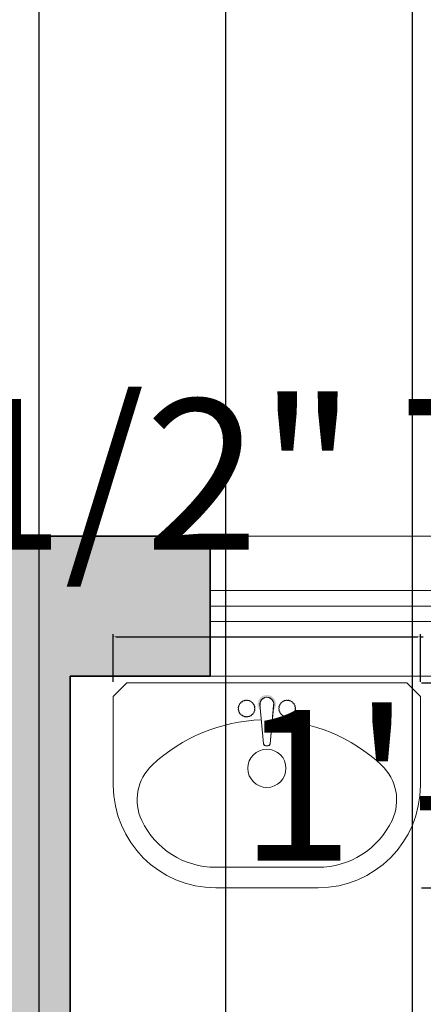
# Model space of a CAD drawing. Units: inches. Extents: x 2103 to 2702, y 2405 to 3142.
# Tile 5 of 7: x 2470 to 2496, y 3039 to 3102. Entities that reach past the tile are written whole.
import ezdxf

# ---------------------------------------------------------------- set-up
doc = ezdxf.new("R2010")
doc.units = ezdxf.units.IN
for name, color, linetype, lineweight in [('A-ANNO-DIMS', 2, 'Continuous', 18), ('A-FLOR-FIXT', 9, 'Continuous', 18), ('A-WALL-PATT', 8, 'Continuous', 9), ('WALL', 7, 'Continuous', 35), ('windows', 4, 'Continuous', 18)]:
    doc.layers.add(name, color=color, linetype=linetype, lineweight=lineweight)
doc.styles.get("Standard").update_dxf_attribs({"font": 'arial.ttf'})
doc.dimstyles.get("Standard").update_dxf_attribs({"dimtxt": 9.68, "dimasz": 0.18, "dimexe": 0.18, "dimexo": 0.0625, "dimgap": 0.09, "dimtad": 0, "dimtih": 1, "dimtoh": 1, "dimdec": 1, "dimzin": 0, "dimdsep": 46, "dimlunit": 3, "dimtxsty": 'Standard', "dimcen": 0.09, "dimadec": 0, "dimazin": 0, "dimtfac": 1, "dimtdec": 1, "dimtofl": 0, "dimtmove": 0, "dimatfit": 3, "dimfxl": 1, "dimtolj": 1, "dimtzin": 0, "dimarcsym": 0})

# ---------------------------------------------------------------- blocks, each defined once
blk = doc.blocks.new('ventilator')
at = {"layer": 'windows'}
for p, q in [((1922.124737122385, 2523.053655013118), (1898.124737122385, 2523.053655013118)), ((1922.124737122385, 2522.053655013118), (1898.124737122385, 2522.053655013118)), ((1922.124737122385, 2521.053655013119), (1898.124737122385, 2521.053655013119))]:
    blk.add_line(p, q, dxfattribs=at)
blk.add_lwpolyline([(1898.124737122385, 2526.553655012885), (1898.124737122385, 2517.553655012886), (1922.124737122385, 2517.553655013119), (1922.124737122385, 2526.553655013119)], close=True, dxfattribs=at)
blk = doc.blocks.new('s_46')
at = {"ltscale": 600}
h = blk.add_hatch(color=256, dxfattribs=at)
edge = h.paths.add_edge_path()
edge.add_line((13.45184378023259, 62.04360352296498), (14.15927104179718, 54.09782096462731))
edge.add_ellipse((4.212458010588306, 52.31250418393756), major_axis=(-10.10576298371302, 2.5e-15), ratio=1, start_angle=540, end_angle=550.1754626554052, ccw=False)
edge.add_arc((4.212458010588306, 52.31250418393756), 10.10576298371302, 270, 360, ccw=False)
edge.add_line((4.212458010588306, 42.20674120020703), (4.212458010588306, 41.28018079043977))
edge.add_line((4.212458010588306, 41.28018079040339), (11.85106942148559, 41.28018079040339))
edge.add_arc((4.212458010588306, 52.31250418393756), 13.41866400745597, 664.6981342835142, 766.4847699121552)
h.paths.add_polyline_path([(4.212458010588306, 41.28018079040339), (-3.426153400272596, 41.28018079040339, 0.152566653256377), (4.212458010588306, 38.8938401764608)])
h.paths.add_polyline_path([(11.85106942144921, 41.28018079040339), (4.212458010588306, 41.28018079040339), (4.212458010588306, 38.8938401764608, 0.1525666532563772)])
h.paths.add_polyline_path([(-5.734355020395014, 54.09782096461277), (-5.026927758881356, 62.04360352296498, 0.4758332592079194), (-3.426153400272596, 41.28018079040339), (4.212458010588306, 41.28018079040339), (4.212458010588306, 42.20674120020703, -0.4672400657637396)])
for p, q in [((-5.893304973142221, 52.31250418385025), (-0.714987907151226, 110.4750654234667)), ((-5.893304973142221, 52.31250418385025), (-0.714987907151226, 110.4750654234667)), ((9.139903928502463, 110.475065423554), (14.15927104174625, 54.09782096461277)), ((14.31822099431883, 52.31250418385025), (9.139903928502463, 110.475065423554)), ((14.15927104174625, 54.09782096461277), (14.31822099431883, 52.31250418385025))]:
    blk.add_line(p, q, dxfattribs=at)
blk.add_lwpolyline([(-220.7875419894117, 171.2801807903452, -0.4142135623730951), (-70.7875419894117, 321.2801807903452), (79.2124580105883, 321.2801807904325, -0.4142135623730951), (229.2124580105883, 171.2801807904325), (229.2124580105883, 41.28018079040339), (209.2124580107047, 21.2801807904325), (-200.7875419893535, 21.28018079034518), (-220.7875419894117, 41.28018079040339)], format="xyb", close=True, dxfattribs=at)
blk.add_lwpolyline([(12.26164246437838, 75.41187665969483, 0.1816379869150311), (172.1859176590806, 141.5383421540609, 0.3263505073803008), (187.6570333366981, 222.6589125997853, 0.2898144196813102), (79.21245801076293, 291.2801807904325), (-70.78754198923707, 291.2801807903452, 0.2898144196813102), (-179.2321173155214, 222.658912599698, 0.3263505073803008), (-163.7610016377293, 141.5383421540609, 0.1816379869150315), (-3.836726442852523, 75.41187665960751)], format="xyb", dxfattribs=at)
for points in [[(-16.83803374727722, 67.43055756771354), (-17.02338931558188, 67.50428807432763), (-17.22058725368697, 67.56961317334208), (-17.42189012444578, 67.6347039079701), (-17.61956049106084, 67.70773132116301), (-17.80586091603618, 67.79686645595939), (-17.97305396257434, 67.91028035557245), (-18.11578784312587, 68.05326030802098), (-18.23825336818117, 68.21955858168076), (-18.34702699835179, 68.40004368982045), (-18.44868519355077, 68.58558414605795), (-18.54980441438965, 68.76704846357461), (-18.65696112113073, 68.9353051558137), (-18.77673177386168, 69.08122273621848), (-18.91569283319404, 69.19566971814493), (-19.07841429975815, 69.27267628890695), (-19.26144033775199, 69.31891933156292), (-19.45930865121772, 69.34423740339116), (-19.66655694507062, 69.35846906132065), (-19.87772292352747, 69.37145286262967), (-20.08734429115429, 69.39302736415993), (-20.2899587523425, 69.43303112310241), (-20.48010401183274, 69.50130269664805), (-20.65391131333308, 69.60429419830325), (-20.81388605764368, 69.73491196823306), (-20.96412718523061, 69.8826759030926), (-21.10873363655992, 70.03710589953698), (-21.25180435174844, 70.18772185422131), (-21.39743827126222, 70.3240436638007), (-21.54973433539272, 70.43559122501756), (-21.71279148443137, 70.5118844343524), (-21.88955151231494, 70.54600451889564), (-22.07832762773614, 70.54527802669325), (-22.27627589285839, 70.52059283622657), (-22.4805523698451, 70.48283682571491), (-22.68831312085968, 70.44289787355228), (-22.89671420806553, 70.41166385821998), (-23.10291169380071, 70.40002265802468), (-23.30406164005399, 70.41886215136037), (-23.49802141042892, 70.4753938675276), (-23.68545357254334, 70.56212393892929), (-23.86772199510597, 70.66788214896224), (-24.04619054717477, 70.78149828102323), (-24.22222309763311, 70.89180211850908), (-24.39718351518968, 70.98762344472925), (-24.57243566872785, 71.05779204316786), (-24.74934342730558, 71.09113769704709), (-24.92903553397628, 71.08022740500746), (-25.11170022917213, 71.03257702605333), (-25.2972906283685, 70.95943963443278), (-25.48575984616764, 70.8720683044812), (-25.67706099752104, 70.7817161102721), (-25.87114719772944, 70.69963612605352), (-26.0679715613951, 70.63708142607356), (-26.26748720381875, 70.60530508466763), (-26.46941223740578, 70.61182491958607), (-26.67252476507565, 70.64921772302478), (-26.87536788737634, 70.70632503094384), (-27.07648470485583, 70.77198837930337), (-27.27441831788747, 70.8350493038015), (-27.46771182701923, 70.88434934031102), (-27.6549083327991, 70.90873002487933), (-27.83455093560042, 70.8970328932919), (-28.00620139669627, 70.84190539614065), (-28.17349611973623, 70.75121864315588), (-28.34109016874572, 70.63664965887438), (-28.51363860827405, 70.50987546765828), (-28.69579650234664, 70.38257309404435), (-28.89221891516354, 70.26641956248204), (-29.10756091127405, 70.17309189750813), (-29.3464775547036, 70.11426712348475), (-29.61160253512208, 70.0940409177856), (-29.89748404390411, 70.0861835690448), (-30.19664889771957, 70.05688401864609), (-30.50162391323829, 69.9723312081478), (-30.80493590747938, 69.79871407902101), (-31.09911169676343, 69.50222157256212), (-31.37667809793493, 69.0490426304168), (-31.63016192783834, 68.40536619405611), (-32.32050594605971, 68.4500712644367), (-32.84873653826071, 68.3918758847285), (-33.24226493795868, 68.25193804170704), (-33.52850237919483, 68.0514157223224), (-33.73486009566113, 67.8114669136994), (-33.88874932087492, 67.5532496026135), (-34.01758128887741, 67.29792177610216), (-34.14876723336056, 67.06664142102818), (-34.30371923936764, 66.87550954936887), (-34.47985279804561, 66.72039927294827), (-34.66858425136889, 66.59212672835565), (-34.86132994201034, 66.48150805244222), (-35.04950621211901, 66.37935938188457), (-35.22452940384392, 66.27649685335928), (-35.37781585985795, 66.16373660371755), (-35.50078192248475, 66.03189476963598), (-35.58785390376579, 65.87432967920904), (-35.64549799636007, 65.69456842611542), (-35.68319036299363, 65.49868029527715), (-35.7104071660433, 65.2927345718781), (-35.73662456823513, 65.08280054092756), (-35.77131873212056, 64.87494748734753), (-35.82396582007641, 64.67524469623459), (-35.90404199482873, 64.48976145259803), (-36.01774371694773, 64.3227640100813), (-36.15814863995183, 64.17130649695173), (-36.31505471485434, 64.0306400101108), (-36.47825989319244, 63.89601564637269), (-36.63756212632871, 63.76268450255157), (-36.78275936545106, 63.62589767554891), (-36.90364956192207, 63.48090626226621), (-36.99003066710429, 63.32296135951764), (-37.03518227743916, 63.14869254492805), (-37.04631056915969, 62.96024331927765), (-37.03410336375237, 62.7611356638954), (-37.00924848217983, 62.55489156045951), (-36.98243374592858, 62.34503299021162), (-36.96434697631048, 62.13508193491725), (-36.96567599463743, 61.92856037581805), (-36.99710862222128, 61.72899029450491), (-37.06570762058254, 61.53896291530691), (-37.16403551277472, 61.35734643402975), (-37.28102976223454, 61.18207828939194), (-37.40562783187488, 61.0110959201993), (-37.52676718513249, 60.84233676508302), (-37.63338528544409, 60.67373826284892), (-37.7144195958972, 60.50323785204091), (-37.75880757992855, 60.32877297155209), (-37.75920177751686, 60.14875038337777), (-37.72311503690435, 59.96345414296957), (-37.66177528270055, 59.77363762940512), (-37.58641044021351, 59.58005422132555), (-37.5082484340528, 59.38345729780849), (-37.43851718935184, 59.18460023758234), (-37.38844463089481, 58.98423641963745), (-37.36925868364051, 58.78311922278953), (-37.38844463089481, 58.58200202594161), (-37.43851718935184, 58.38163820799673), (-37.5082484340528, 58.18278114777058), (-37.58641044021351, 57.98618422425352), (-37.66177528287517, 57.79260081626126), (-37.72311503690435, 57.6027843026095), (-37.75920177751686, 57.4174880622013), (-37.75880757992855, 57.23746547402697), (-37.7144195958972, 57.06300059353816), (-37.63338528544409, 56.89250018273014), (-37.52676718530711, 56.72390168049606), (-37.40562783187488, 56.55514252537978), (-37.28102976223454, 56.38416015618713), (-37.16403551277472, 56.20889201154932), (-37.06570762058254, 56.02727553035947), (-36.99710862222128, 55.83724815107416), (-36.96567599463743, 55.63767806976102), (-36.96434697631048, 55.43115651066182), (-36.98243374592858, 55.22120545536745), (-37.00924848217983, 55.01134688520687), (-37.03410336375237, 54.80510278168367), (-37.04631056933431, 54.60599512638873), (-37.03518227743916, 54.41754590065102), (-36.99003066710429, 54.24327708606142), (-36.90364956192207, 54.08533218331285), (-36.78275936545106, 53.94034077003016), (-36.63756212632871, 53.80355394302751), (-36.47825989319244, 53.67022279920639), (-36.31505471502896, 53.53559843546827), (-36.15814863995183, 53.39493194862734), (-36.01774371712236, 53.24347443549777), (-35.90404199482873, 53.07647699298104), (-35.82396582007641, 52.89099374934449), (-35.77131873212056, 52.69129095823155), (-35.73662456823513, 52.48343790465151), (-35.71040716621792, 52.27350387370098), (-35.68319036299363, 52.06755815021461), (-35.64549799653469, 51.87167001946363), (-35.58785390376579, 51.69190876637003), (-35.50078192248475, 51.53434367594309), (-35.3778353385278, 51.40284301002975), (-35.22468523163116, 51.29247093791491), (-35.05003213009331, 51.19609060572111), (-34.86257656256203, 51.10656515930895), (-34.67101905716118, 51.01675774488831), (-34.48406014236389, 50.91953150840708), (-34.31040034646867, 50.80774959607516), (-34.15874019777402, 50.67427515375311), (-34.03505195630714, 50.51453334218241), (-33.93439480883535, 50.3341973797942), (-33.84909967368003, 50.14150249981321), (-33.77149746881332, 49.94468393520219), (-33.69391911290586, 49.75197691909852), (-33.60869552427903, 49.57161668455228), (-33.50815762107959, 49.41183846470085), (-33.38463632145431, 49.28087749250699), (-33.23284944484476, 49.18408373402781), (-33.05706241185544, 49.11526608630083), (-32.86392754490953, 49.06534817945794), (-32.66009716555709, 49.02525364354369), (-32.45222359569743, 48.98590610860265), (-32.24695915722987, 48.93822920459206), (-32.05095617187908, 48.87314656155649), (-31.870866961719, 48.78158180962782), (-31.71133844077122, 48.65761859554914), (-31.5689958925941, 48.50798063381808), (-31.43845919286832, 48.34255165536887), (-31.31434821744915, 48.17121539139771), (-31.19128284219187, 48.00385557310073), (-31.06388294277713, 47.85035593167413), (-30.92676839523483, 47.72060019822674), (-30.77455907507101, 47.62447210386745), (-30.60346923320321, 47.56846716045401), (-30.41609062027419, 47.54552800310193), (-30.21660936163971, 47.54520904741366), (-30.00921158283018, 47.55706470907898), (-29.79808340937598, 47.570649403875), (-29.58741096680751, 47.57551754757878), (-29.38138038065517, 47.56122355579281), (-29.18417777627474, 47.51732184420689), (-28.99883273948217, 47.43692629240103), (-28.8237486963626, 47.32738863455597), (-28.65617253311211, 47.19962006882997), (-28.49335113610141, 47.06453179311938), (-28.33253139152657, 46.9330350055825), (-28.1709601857583, 46.81604090429027), (-28.00588440499268, 46.72446068713907), (-27.83455093577504, 46.66920555219985), (-27.6549083327991, 46.65750842061243), (-27.46771182701923, 46.68188910518074), (-27.27441831788747, 46.73118914177758), (-27.07648470485583, 46.7942500662757), (-26.87536788755096, 46.85991341454792), (-26.67252476525027, 46.91702072246698), (-26.4694122375804, 46.95441352590569), (-26.26748720399337, 46.96093336082412), (-26.06797156156972, 46.9291570194182), (-25.87114719772944, 46.86660231943824), (-25.67706099769566, 46.78452233530697), (-25.48575984616764, 46.69417014101054), (-25.2972906283685, 46.60679881105898), (-25.11170022934675, 46.53366141943843), (-24.92903553397628, 46.4860110404843), (-24.74934342730558, 46.47510074844467), (-24.57243566890247, 46.50844640232389), (-24.39718351536431, 46.57861500076251), (-24.22222309780773, 46.67443632698268), (-24.0461905473494, 46.78474016446853), (-23.86772199528059, 46.89835629652953), (-23.68545357254334, 47.00411450656247), (-23.49802141060354, 47.09084457796416), (-23.30406164022861, 47.14737629413138), (-23.10291169380071, 47.16621578746708), (-22.89671420806553, 47.15457458727178), (-22.68831312085968, 47.12334057193948), (-22.4805523698451, 47.08340161977685), (-22.27627589285839, 47.04564560926519), (-22.07832762791077, 47.02096041871118), (-21.88955151248956, 47.02023392650881), (-21.71279148443137, 47.05435401113937), (-21.54973433539272, 47.1306472204742), (-21.39743827126222, 47.24219478160375), (-21.25180435174844, 47.37851659118314), (-21.10873363655992, 47.52913254586746), (-20.96412718540523, 47.68356254231185), (-20.81388605764368, 47.83132647717138), (-20.65391131333308, 47.9619442471012), (-20.48010401200736, 48.0649357488437), (-20.28995875251712, 48.13320732230204), (-20.08734429115429, 48.17321108133183), (-19.87772292352747, 48.1947855828621), (-19.66655694507062, 48.2077693840838), (-19.45930865139235, 48.2220010421006), (-19.26144033775199, 48.24731911384152), (-19.07841429993277, 48.29356215667212), (-18.91569283319404, 48.37056872743414), (-18.77673177403631, 48.48501570936059), (-18.65696112113073, 48.63093328976538), (-18.54980441456428, 48.79918998200446), (-18.44868519372539, 48.98065429960843), (-18.34702699835179, 49.16619475575862), (-18.2382533683558, 49.34667986398562), (-18.11578784312587, 49.5129781376454), (-17.97305396274896, 49.6559580900066), (-17.8058609162108, 49.76937198961969), (-17.61956049106084, 49.85850712450337), (-17.4218901246204, 49.93153453769628), (-17.22058725368697, 49.996625272237), (-17.02338931558188, 50.06195037133875), (-16.83803374727722, 50.13568087795284), (-16.67225798609434, 50.22598783511785), (-16.53379946883069, 50.34104228604701), (-16.42766593385022, 50.48645191569812), (-16.34794632298872, 50.65757097714231), (-16.28599987912457, 50.84719036528259), (-16.23318584513618, 51.04810097528389), (-16.18086346407654, 51.25309370196191), (-16.12039197882404, 51.45495944039431), (-16.04313063243171, 51.64648908557137), (-15.94043866742868, 51.82047353248345), (-15.8067031877581, 51.97190354572376), (-15.64842273970134, 52.10456936812261), (-15.47512373042991, 52.22446111202589), (-15.29633256676607, 52.33756888969219), (-15.12157565605594, 52.44988281364204), (-14.96037940529641, 52.567392996134), (-14.82227022130973, 52.69608954960131), (-14.71677451161667, 52.84196258638985), (-14.6501372611965, 53.00919824198354), (-14.61547776852967, 53.19476674450561), (-14.60263391025364, 53.3938343450427), (-14.60144356318051, 53.60156729485606), (-14.60174460412236, 53.81313184503233), (-14.59337490954203, 54.02369424700736), (-14.566172356077, 54.22842075169319), (-14.50997482053935, 54.42247761052567), (-14.41809999983525, 54.6024088327249), (-14.29778487142175, 54.77026946117985), (-14.1597462335485, 54.92949229647638), (-14.01470088359201, 55.08351013963693), (-13.87336561962729, 55.23575579150929), (-13.7464572393801, 55.38966205302859), (-13.64469254092546, 55.54866172495531), (-13.5787883218145, 55.71618760822457), (-13.55583441938506, 55.89474125843844), (-13.56841282837558, 56.08309925056528), (-13.60547858278733, 56.27910691397847), (-13.65598671662155, 56.48060957840062), (-13.70889226370491, 56.68545257346704), (-13.7531502583879, 56.89148122872575), (-13.7777157346718, 57.09654087381204), (-13.77154372638324, 57.29847683827393), (-13.72730239736847, 57.49560352915432), (-13.65251243085367, 57.68811166286468), (-13.55840763938613, 57.8766610333987), (-13.45622183586238, 58.06191143448813), (-13.35718883317895, 58.24452266012667), (-13.27254244388314, 58.42515450413339), (-13.2135164810461, 58.60446676041465), (-13.19134475721512, 58.78311922278953), (-13.2135164810461, 58.96177168516442), (-13.27254244388314, 59.14108394144569), (-13.35718883317895, 59.3217157854524), (-13.45622183586238, 59.50432701109093), (-13.55840763938613, 59.68957741218037), (-13.65251243085367, 59.87812678271438), (-13.72730239736847, 60.07063491642475), (-13.77154372638324, 60.26776160730515), (-13.7777157346718, 60.46969757176703), (-13.7531502583879, 60.67475721685332), (-13.70889226370491, 60.88078587211203), (-13.65598671662155, 61.08562886717845), (-13.60547858278733, 61.2871315316006), (-13.56841282837558, 61.48313919501379), (-13.55583441938506, 61.67149718714063), (-13.5787883218145, 61.8500508373545), (-13.64469254092546, 62.01757672062377), (-13.7464572393801, 62.17657639255048), (-13.87336561962729, 62.33048265406978), (-14.01470088359201, 62.48272830594214), (-14.15974623337388, 62.63674614910269), (-14.29778487142175, 62.79596898448653), (-14.41809999983525, 62.96382961285416), (-14.50997482053935, 63.14376083514071), (-14.566172356077, 63.33781769388588), (-14.59337490936741, 63.5425441985717), (-14.60174460412236, 63.75310660054674), (-14.60144356318051, 63.96467115081032), (-14.60263391025364, 64.17240410053635), (-14.61547776835505, 64.37147170116077), (-14.65013726102188, 64.55704020359553), (-14.71677451144205, 64.7242758591892), (-14.82227022130973, 64.87014889597776), (-14.96037940529641, 64.99884544944507), (-15.12157565605594, 65.11635563193704), (-15.29633256676607, 65.22866955588688), (-15.47512373042991, 65.3417773336405), (-15.64842273970134, 65.46166907745646), (-15.8067031877581, 65.59433489985531), (-15.94043866742868, 65.74576491309563), (-16.04313063225709, 65.9197493600077), (-16.12039197882404, 66.11127900527208), (-16.18086346407654, 66.31314474370447), (-16.23318584513618, 66.5181374703825), (-16.28599987912457, 66.71904808029649), (-16.34794632298872, 66.90866746843676), (-16.42766593385022, 67.07978652988095), (-16.53379946883069, 67.22519615953206), (-16.67225798609434, 67.34025061046123)], [(22.08090273779817, 61.08562886709115), (22.03039460413856, 61.2871315315133), (21.99332884972682, 61.48313919501379), (21.9807504407363, 61.67149718705331), (22.00370434316574, 61.85005083726719), (22.06960856210208, 62.01757672053645), (22.17137326073134, 62.17657639246318), (22.29828164080391, 62.33048265398247), (22.43961690476863, 62.48272830585483), (22.58466225472512, 62.63674614901538), (22.72270089277299, 62.79596898439923), (22.84301602118649, 62.96382961276686), (22.93489084189059, 63.1437608350534), (22.99108837742824, 63.33781769379857), (23.01829093071865, 63.5425441985717), (23.0266606254736, 63.75310660045943), (23.02635958453175, 63.96467115072301), (23.02754993160488, 64.17240410053635), (23.04039378970629, 64.37147170107346), (23.07505328237312, 64.55704020350822), (23.14169053279329, 64.72427585910191), (23.24718624266097, 64.87014889589045), (23.38529542664764, 64.99884544935776), (23.54649167740717, 65.11635563193704), (23.7212485881173, 65.22866955579956), (23.90003975178115, 65.34177733355318), (24.07333876105258, 65.46166907736915), (24.23161920910934, 65.594334899768), (24.36535468877992, 65.74576491300832), (24.46804665360833, 65.9197493600077), (24.54530800017528, 66.11127900518477), (24.60577948542777, 66.31314474361714), (24.65810186648742, 66.51813747029519), (24.71091590047581, 66.71904808020918), (24.77286234433996, 66.90866746834945), (24.85258195520146, 67.07978652979364), (24.95871549018193, 67.22519615953206), (25.09717400744558, 67.34025061046123), (25.26294976862846, 67.43055756771354), (25.44830533693312, 67.50428807432763), (25.64550327503821, 67.56961317334208), (25.84680614579702, 67.6347039079701), (26.04447651241208, 67.70773132116301), (26.23077693756204, 67.79686645595939), (26.3979699841002, 67.91028035557245), (26.54070386447711, 68.05326030802098), (26.66316938970704, 68.21955858168076), (26.77194301970303, 68.40004368982045), (26.87360121507663, 68.58558414605795), (26.97472043591552, 68.76704846357461), (27.08187714248197, 68.9353051558137), (27.20164779538754, 69.08122273621848), (27.34060885454528, 69.19566971814493), (27.50333032128401, 69.27267628890695), (27.68635635910323, 69.31891933165025), (27.88422467274358, 69.34423740347847), (28.09147296642186, 69.35846906140794), (28.30263894487871, 69.37145286262967), (28.51226031250553, 69.39302736424725), (28.71487477386836, 69.43303112318972), (28.90502003318398, 69.50130269673537), (29.07882733468432, 69.60429419839056), (29.23880207899492, 69.73491196832038), (29.38904320658185, 69.88267590317992), (29.53364965791116, 70.0371058996243), (29.67672037309967, 70.18772185430862), (29.82235429261346, 70.324043663888), (29.97465035674395, 70.43559122501756), (30.1377075057826, 70.51188443443971), (30.31446753366618, 70.54600451898295), (30.50324364908738, 70.54527802678058), (30.70119191420963, 70.52059283622657), (30.90546839119634, 70.48283682571491), (31.11322914221091, 70.4428978736396), (31.32163022941677, 70.41166385830729), (31.52782771515195, 70.400022658112), (31.72897766157985, 70.41886215144768), (31.92293743178016, 70.4753938675276), (32.11036959389458, 70.56212393892929), (32.29263801663183, 70.66788214896224), (32.47110656870063, 70.78149828102323), (32.64713911898434, 70.89180211850908), (32.82209953654092, 70.98762344481656), (32.99735169025371, 71.05779204316786), (33.17425944865681, 71.09113769704709), (33.35395155532751, 71.08022740500746), (33.53661625069799, 71.03257702605333), (33.72220664971974, 70.9594396345201), (33.91067586751888, 70.8720683044812), (34.1019770190469, 70.7817161102721), (34.29606321908068, 70.69963612605352), (34.49288758292096, 70.63708142616088), (34.69240322534461, 70.60530508466763), (34.89432825893164, 70.61182491958607), (35.09744078660151, 70.64921772302478), (35.3002839089022, 70.70632503103116), (35.50140072620707, 70.77198837930337), (35.6993343392387, 70.8350493038015), (35.89262784837047, 70.88434934039833), (36.07982435415034, 70.90873002487933), (36.25946695695166, 70.8970328932919), (36.43111741804751, 70.84190539614065), (36.59841214108747, 70.75121864315588), (36.76600619009696, 70.63664965887438), (36.93855462962529, 70.50987546765828), (37.12071252369788, 70.38257309404435), (37.3171349366894, 70.26641956248204), (37.53247693262529, 70.17309189750813), (37.77139357605483, 70.11426712348475), (38.03651855647331, 70.0940409177856), (38.32240006525535, 70.0861835690448), (38.62156491907081, 70.05688401864609), (38.92653993476415, 69.9723312081478), (39.22985192883061, 69.79871407893368), (39.52402771811467, 69.50222157256212), (39.80159411928616, 69.0490426304168), (40.05507794918957, 68.4053661939688), (40.74542196741094, 68.4500712644367), (41.27365255961194, 68.3918758846412), (41.66718095948453, 68.25193804161972), (41.95341840054607, 68.0514157223224), (42.15977611701236, 67.8114669136121), (42.31366534240078, 67.5532496025262), (42.44249731022864, 67.29792177601485), (42.57368325471179, 67.06664142094087), (42.72863526071887, 66.87550954936887), (42.90476881939684, 66.72039927286096), (43.09350027272012, 66.59212672826834), (43.28624596336157, 66.48150805235491), (43.47442223347025, 66.37935938179726), (43.64944542536977, 66.27649685335928), (43.80273188138381, 66.16373660371755), (43.92569794383598, 66.03189476963598), (44.01276992511703, 65.87432967912173), (44.0704140177113, 65.69456842602813), (44.10810638434486, 65.49868029527715), (44.13532318739453, 65.2927345718781), (44.16154058958636, 65.08280054084025), (44.19623475347179, 64.87494748726021), (44.24888184142765, 64.67524469614727), (44.32895801617997, 64.48976145251072), (44.44265973829897, 64.32276400999397), (44.58306466130307, 64.17130649695173), (44.73997073620558, 64.03064001002348), (44.90317591454368, 63.89601564628538), (45.06247814767994, 63.76268450246425), (45.20767538680229, 63.6258976754616), (45.3285655832733, 63.4809062621789), (45.41494668845553, 63.32296135943034), (45.46009829879039, 63.14869254484074), (45.47122659051092, 62.96024331919034), (45.45901938492898, 62.76113566380809), (45.43416450353106, 62.5548915603722), (45.40734976727981, 62.34503299021162), (45.38926299766171, 62.13508193482994), (45.39059201598866, 61.92856037573074), (45.42202464357251, 61.7289902944176), (45.49062364193377, 61.53896291521959), (45.58895153412595, 61.35734643394243), (45.70594578341115, 61.18207828939194), (45.83054385322611, 61.01109592011198), (45.95168320648371, 60.84233676508302), (46.05830130679533, 60.67373826276162), (46.13933561724843, 60.50323785204091), (46.18372360127978, 60.32877297146479), (46.1841177988681, 60.14875038329046), (46.14803105825558, 59.96345414296957), (46.08669130405178, 59.77363762931782), (46.01132646156474, 59.58005422123824), (45.93316445540404, 59.38345729772118), (45.86343321070308, 59.18460023749503), (45.81336065224604, 58.98423641955014), (45.79417470499175, 58.78311922270222), (45.81336065224604, 58.58200202585431), (45.86343321070308, 58.38163820790942), (45.93316445540404, 58.18278114777058), (46.01132646156474, 57.98618422416621), (46.08669130405178, 57.79260081617394), (46.14803105808095, 57.6027843025222), (46.1841177988681, 57.4174880622013), (46.18372360127978, 57.23746547393966), (46.13933561724843, 57.06300059345085), (46.05830130679533, 56.89250018273014), (45.95168320648371, 56.72390168040874), (45.83054385322611, 56.55514252529247), (45.70594578341115, 56.38416015609982), (45.58895153412595, 56.20889201154932), (45.49062364193377, 56.02727553027216), (45.42202464339789, 55.83724815107416), (45.39059201598866, 55.63767806976102), (45.38926299766171, 55.43115651066182), (45.40734976727981, 55.22120545528014), (45.43416450335644, 55.01134688511957), (45.45901938492898, 54.80510278159636), (45.47122659051092, 54.60599512630142), (45.46009829879039, 54.41754590056371), (45.41494668845553, 54.24327708597411), (45.32856558309868, 54.08533218322554), (45.20767538662767, 53.94034076994285), (45.06247814750532, 53.8035539429402), (44.90317591454368, 53.67022279920639), (44.73997073620558, 53.53559843538096), (44.58306466130307, 53.39493194854004), (44.44265973829897, 53.24347443541046), (44.32895801617997, 53.07647699298104), (44.24888184125302, 52.89099374934449), (44.19623475329717, 52.69129095823155), (44.16154058958636, 52.48343790465151), (44.13532318739453, 52.27350387361366), (44.10810638434486, 52.06755815021461), (44.0704140177113, 51.87167001946363), (44.01276992511703, 51.69190876628272), (43.92569794366136, 51.53434367585578), (43.80275135970442, 51.40284301002975), (43.64960125280776, 51.29247093791491), (43.47494815144455, 51.1960906056338), (43.28749258373863, 51.10656515922165), (43.09593507851241, 51.01675774480099), (42.90897616371512, 50.91953150840708), (42.73531636764528, 50.80774959598784), (42.58365621895063, 50.67427515375311), (42.45996797765838, 50.51453334218241), (42.35931083018658, 50.3341973797942), (42.27401569485664, 50.14150249981321), (42.19641349016455, 49.94468393520219), (42.1188351342571, 49.75197691909852), (42.03361154545564, 49.57161668455228), (41.9330736422562, 49.41183846461354), (41.80955234280554, 49.28087749250699), (41.65776546602137, 49.1840837339405), (41.48197843320668, 49.11526608630083), (41.28884356608614, 49.06534817945794), (41.0850131867337, 49.02525364354369), (40.87713961687405, 48.98590610851534), (40.67187517840648, 48.93822920459206), (40.47587219323031, 48.87314656155649), (40.29578298289561, 48.78158180962782), (40.13625446194782, 48.65761859554914), (39.99391191377072, 48.50798063373076), (39.86337521404493, 48.34255165528157), (39.73926423862577, 48.17121539139771), (39.61619886336848, 48.00385557310073), (39.48879896395374, 47.85035593167413), (39.35168441641144, 47.72060019813944), (39.19947509624762, 47.62447210378013), (39.02838525455445, 47.56846716045401), (38.8410066414508, 47.54552800310193), (38.64152538281633, 47.54520904732635), (38.43412760400679, 47.55706470907898), (38.22299943072721, 47.570649403875), (38.01232698798413, 47.57551754757878), (37.80629640183179, 47.56122355579281), (37.60909379745135, 47.51732184420689), (37.42374876065878, 47.43692629240103), (37.24866471753922, 47.32738863455597), (37.08108855428873, 47.19962006882997), (36.91826715727803, 47.06453179311938), (36.75744741270319, 46.9330350056698), (36.59587620693492, 46.81604090429027), (36.4308004261693, 46.72446068713907), (36.25946695695166, 46.66920555228716), (36.07982435397571, 46.65750842061243), (35.89262784837047, 46.68188910518074), (35.6993343392387, 46.73118914177758), (35.50140072620707, 46.7942500662757), (35.30028390872758, 46.85991341454792), (35.09744078642689, 46.91702072246698), (34.89432825875701, 46.954413525993), (34.69240322516998, 46.96093336082412), (34.49288758274633, 46.9291570194182), (34.29606321908068, 46.86660231943824), (34.10197701887228, 46.78452233530697), (33.91067586734425, 46.69417014109785), (33.72220664971974, 46.60679881105898), (33.53661625052337, 46.53366141943843), (33.35395155515289, 46.4860110404843), (33.17425944865681, 46.47510074844467), (32.99735169007909, 46.5084464024112), (32.82209953654092, 46.57861500076251), (32.64713911898434, 46.67443632707), (32.47110656852601, 46.78474016446853), (32.2926380164572, 46.89835629661684), (32.11036959389458, 47.00411450664979), (31.92293743178016, 47.09084457805147), (31.72897766140522, 47.14737629413138), (31.52782771497732, 47.16621578746708), (31.32163022941677, 47.15457458727178), (31.11322914203629, 47.12334057193948), (30.90546839102171, 47.08340161986416), (30.70119191420963, 47.0456456093525), (30.50324364908738, 47.02096041879849), (30.31446753366618, 47.02023392659611), (30.1377075057826, 47.05435401113937), (29.97465035674395, 47.13064722056151), (29.82235429261346, 47.24219478169106), (29.67672037309967, 47.37851659127045), (29.53364965791116, 47.52913254595478), (29.38904320658185, 47.68356254239916), (29.2388020788203, 47.8313264772587), (29.0788273345097, 47.96194424718851), (28.90502003318398, 48.06493574893102), (28.71487477369374, 48.13320732238935), (28.51226031250553, 48.17321108133183), (28.30263894487871, 48.19478558294941), (28.09147296642186, 48.20776938417111), (27.88422467256896, 48.22200104218791), (27.68635635892861, 48.24731911392882), (27.50333032110939, 48.29356215667212), (27.34060885454528, 48.37056872743414), (27.20164779521292, 48.48501570936059), (27.08187714248197, 48.63093328976538), (26.97472043574089, 48.79918998200446), (26.87360121490201, 48.98065429960843), (26.77194301952841, 49.16619475575862), (26.66316938953241, 49.34667986398562), (26.54070386447711, 49.51297813755809), (26.39796998392558, 49.6559580900066), (26.23077693738742, 49.76937198961969), (26.04447651223745, 49.85850712450337), (25.84680614579702, 49.93153453769628), (25.64550327486359, 49.996625272237), (25.44830533675849, 50.06195037133875), (25.26294976862846, 50.13568087795284), (25.09717400727095, 50.22598783520516), (24.95871549018193, 50.34104228604701), (24.85258195520146, 50.48645191561082), (24.77286234416534, 50.657570977055), (24.71091590030119, 50.84719036519527), (24.65810186648742, 51.04810097519657), (24.60577948542777, 51.2530937018746), (24.54530800017528, 51.45495944030699), (24.46804665360833, 51.64648908548406), (24.36535468877992, 51.82047353239614), (24.23161920910934, 51.97190354572376), (24.07333876105258, 52.1045693680353), (23.90003975160653, 52.22446111193858), (23.7212485881173, 52.33756888960488), (23.54649167740717, 52.44988281355472), (23.38529542647302, 52.56739299604669), (23.24718624266097, 52.696089549514), (23.14169053279329, 52.84196258630254), (23.07505328237312, 53.00919824189623), (23.04039378970629, 53.1947667444183), (23.02754993160488, 53.39383434495539), (23.02635958453175, 53.60156729476876), (23.02666062529898, 53.81313184503233), (23.01829093071865, 54.02369424692006), (22.99108837725362, 54.22842075169319), (22.93489084171597, 54.42247761043836), (22.84301602101186, 54.6024088327249), (22.72270089277299, 54.77026946109254), (22.58466225472512, 54.92949229638907), (22.43961690476863, 55.08351013963693), (22.29828164080391, 55.23575579150929), (22.17137326073134, 55.38966205294127), (22.06960856210208, 55.548661724868), (22.00370434316574, 55.71618760813726), (21.9807504407363, 55.89474125843844), (21.99332884972682, 56.08309925047797), (22.03039460413856, 56.27910691389115), (22.08090273779817, 56.48060957840062), (22.13380828505615, 56.68545257346704), (22.17806627973914, 56.89148122872575), (22.20263175602304, 57.09654087381204), (22.19645974773448, 57.29847683827393), (22.15221841871971, 57.49560352915432), (22.07742845220491, 57.68811166286468), (21.98332366073737, 57.87666103331139), (21.88113785721362, 58.06191143448813), (21.78210485453019, 58.24452266012667), (21.69745846523438, 58.42515450413339), (21.63843250239734, 58.60446676032734), (21.61626077856636, 58.78311922270222), (21.63843250239734, 58.96177168507711), (21.69745846523438, 59.14108394135837), (21.78210485453019, 59.32171578536508), (21.88113785721362, 59.50432701100362), (21.98332366073737, 59.68957741209306), (22.07742845220491, 59.87812678262708), (22.15221841871971, 60.07063491633743), (22.19645974773448, 60.26776160721784), (22.20263175602304, 60.46969757167971), (22.17806627973914, 60.67475721676601), (22.13380828505615, 60.88078587202471)]]:
    blk.add_lwpolyline(points, close=True, dxfattribs=at)
blk.add_circle((4.212458010588306, 146.2801807904034), 28, dxfattribs=at)
for centre, radius, start, end in [((4.212458010588306, 108.2109541267855), 5.422722861947412, 24.67830004152974, 155.3216999584702), ((4.212458010588306, 52.31250418393756), 10.10576298371233, 169.8245373479931, 0)]:
    blk.add_arc(centre, radius, start, end, dxfattribs=at)
for centre, major_axis, ratio, start_param, end_param in [((4.212458010762929, 110.475065423554), (-4.927445917859709, 1.2e-15), 0.6410240960233505, 3.141592653589793, 6.283185307179586), ((4.212458010588306, 52.31250418393756), (-10.10576298371302, 2.5e-15), 1, 6.105589980929039, 9.602373287019926)]:
    blk.add_ellipse(centre, major_axis=major_axis, ratio=ratio, start_param=start_param, end_param=end_param, dxfattribs=at)
blk = doc.blocks.new('*D15')
at = {"layer": 'A-ANNO-DIMS', "color": 0, "lineweight": -2, "transparency": 16777216}
for p, q in [((2246.430135310188, 3068.908174366427), (2246.430135310188, 3136.18297836625)), ((2246.610135310187, 3136.002978366251), (2418.129303113734, 3136.002978366251)), ((2606.250135310188, 3136.002978366251), (2434.730967506641, 3136.002978366251)), ((2606.430135310187, 3068.908174366427), (2606.430135310187, 3136.18297836625))]:
    blk.add_line(p, q, dxfattribs=at)
at = {"layer": 'A-ANNO-DIMS', "color": 0, "transparency": 16777216}
for points in [[(2246.610135310187, 3136.032978366251), (2246.610135310187, 3135.97297836625), (2246.430135310188, 3136.002978366251)], [(2606.250135310188, 3136.032978366251), (2606.250135310188, 3135.97297836625), (2606.430135310187, 3136.002978366251)]]:
    blk.add_solid(points, dxfattribs=at)
at = {"layer": 'Defpoints', "color": 0, "transparency": 16777216}
for p in [(2606.430135310187, 3136.002978366251), (2246.430135310188, 3068.845674366427), (2606.430135310187, 3068.845674366427)]:
    blk.add_point(p, dxfattribs=at)
at = {"layer": 'A-ANNO-DIMS', "color": 0, "transparency": 16777216, "insert": (2426.430135310188, 3136.002978366251), "char_height": 9.68, "attachment_point": 5}
blk.add_mtext("\\A1;30'", dxfattribs=at)
blk = doc.blocks.new('*D32')
at = {"layer": 'A-ANNO-DIMS', "color": 0, "lineweight": -2, "transparency": 16777216}
for p, q in [((2523.701954441973, 3069.816092044852), (2527.298623542507, 3072.777740503555)), ((2527.0452500719, 3072.802273835842), (2526.8652500719, 3072.802273835842)), ((2527.15967014106, 3072.663320434396), (2527.0452500719, 3072.802273835842)), ((2546.291633940058, 3049.429184449692), (2527.274090210219, 3072.524367032949)), ((2542.948338310131, 3046.443002658702), (2546.545007410664, 3049.404651117404))]:
    blk.add_line(p, q, dxfattribs=at)
at = {"layer": 'A-ANNO-DIMS', "color": 0, "transparency": 16777216}
for points in [[(2527.297249110461, 3072.543437044476), (2527.250931309978, 3072.505297021422), (2527.15967014106, 3072.663320434396)], [(2546.3147928403, 3049.448254461218), (2546.268475039817, 3049.410114438165), (2546.406054009218, 3049.290231048245)]]:
    blk.add_solid(points, dxfattribs=at)
at = {"layer": 'Defpoints', "color": 0, "transparency": 16777216}
for p in [(2527.15967014106, 3072.663320434396), (2523.653706733137, 3069.776362854172), (2542.900090601295, 3046.403273468022)]:
    blk.add_point(p, dxfattribs=at)
at = {"layer": 'A-ANNO-DIMS', "color": 0, "transparency": 16777216, "insert": (2430.028074082815, 3072.802273835842), "char_height": 9.68, "attachment_point": 5}
blk.add_mtext('\\A1;SINK ENVELOPE 2\'-6 1/2" TYP.', dxfattribs=at)
blk = doc.blocks.new('*D38')
at = {"layer": 'A-ANNO-DIMS', "color": 0, "lineweight": -2, "transparency": 16777216}
for p, q in [((2476.201427045263, 3059.468199006091), (2476.201427045263, 3062.547546711256)), ((2495.947078413032, 3059.468199006091), (2495.947078413032, 3062.547546711256)), ((2476.381427045263, 3062.367546711256), (2495.767078413031, 3062.367546711256)), ((2495.947078413032, 3062.367546711256), (2496.127078413031, 3062.367546711256))]:
    blk.add_line(p, q, dxfattribs=at)
at = {"layer": 'A-ANNO-DIMS', "color": 0, "transparency": 16777216}
for points in [[(2476.381427045263, 3062.397546711256), (2476.381427045263, 3062.337546711256), (2476.201427045263, 3062.367546711256)], [(2495.767078413031, 3062.397546711256), (2495.767078413031, 3062.337546711256), (2495.947078413032, 3062.367546711256)]]:
    blk.add_solid(points, dxfattribs=at)
at = {"layer": 'Defpoints', "color": 0, "transparency": 16777216}
for p in [(2495.947078413032, 3062.367546711256), (2476.201427045263, 3059.405699006091), (2495.947078413032, 3059.405699006091)]:
    blk.add_point(p, dxfattribs=at)
at = {"layer": 'A-ANNO-DIMS', "color": 0, "transparency": 16777216, "insert": (2542.315932437588, 3062.367546711256), "char_height": 9.68, "attachment_point": 5}
blk.add_mtext('\\A1;BASIN 1\'-7 1/2"', dxfattribs=at)
blk = doc.blocks.new('*D39')
at = {"layer": 'A-ANNO-DIMS', "color": 0, "lineweight": -2, "transparency": 16777216}
for p, q in [((2496.009578413032, 3059.405699006092), (2499.088926118198, 3059.405699006092)), ((2498.908926118199, 3059.225699006092), (2498.908926118199, 3057.773624220927)), ((2498.908926118199, 3046.421931427576), (2498.908926118199, 3047.874006212741)), ((2496.009578413032, 3046.241931427576), (2499.088926118198, 3046.241931427576))]:
    blk.add_line(p, q, dxfattribs=at)
at = {"layer": 'A-ANNO-DIMS', "color": 0, "transparency": 16777216}
for points in [[(2498.878926118198, 3059.225699006092), (2498.938926118199, 3059.225699006092), (2498.908926118199, 3059.405699006092)], [(2498.878926118198, 3046.421931427576), (2498.938926118199, 3046.421931427576), (2498.908926118199, 3046.241931427576)]]:
    blk.add_solid(points, dxfattribs=at)
at = {"layer": 'Defpoints', "color": 0, "transparency": 16777216}
for p in [(2495.947078413032, 3059.405699006092), (2495.947078413032, 3046.241931427576), (2498.908926118199, 3046.241931427576)]:
    blk.add_point(p, dxfattribs=at)
at = {"layer": 'A-ANNO-DIMS', "color": 0, "transparency": 16777216, "insert": (2498.908926118199, 3052.823815216833), "char_height": 9.68, "attachment_point": 5}
blk.add_mtext('\\A1;1\'-1"', dxfattribs=at)
blk = doc.blocks.new('*D44')
at = {"layer": 'A-ANNO-DIMS', "color": 0, "lineweight": -2, "transparency": 16777216}
for p, q in [((2471.430135, 2560.908174), (2471.430135, 3118.895223)), ((2483.430135, 2560.908174), (2483.430135, 3118.895223)), ((2471.610135, 3118.715223000001), (2483.250135, 3118.715223000001)), ((2483.430135, 3118.715223000001), (2483.610135, 3118.715223000001))]:
    blk.add_line(p, q, dxfattribs=at)
at = {"layer": 'A-ANNO-DIMS', "color": 0, "transparency": 16777216}
for points in [[(2471.610135, 3118.745223000001), (2471.610135, 3118.685223), (2471.430135, 3118.715223000001)], [(2483.250135, 3118.745223000001), (2483.250135, 3118.685223), (2483.430135, 3118.715223000001)]]:
    blk.add_solid(points, dxfattribs=at)
at = {"layer": 'Defpoints', "color": 0, "transparency": 16777216}
for p in [(2483.430135, 3118.715223000001), (2471.430135, 2560.845674), (2483.430135, 2560.845674)]:
    blk.add_point(p, dxfattribs=at)
at = {"layer": 'A-ANNO-DIMS', "color": 0, "transparency": 16777216, "insert": (2496.11047606412, 3118.715223000001), "char_height": 9.68, "attachment_point": 5}
blk.add_mtext('\\A1;1\'-0"', dxfattribs=at)
blk = doc.blocks.new('*D50')
at = {"layer": 'A-ANNO-DIMS', "color": 0, "lineweight": -2, "transparency": 16777216}
for p, q in [((2453.430135, 2569.908174), (2453.430135, 3118.895223)), ((2495.430135, 2569.908174), (2495.430135, 3118.895223)), ((2453.610135, 3118.715223000001), (2461.477488342429, 3118.715223000001)), ((2495.250135, 3118.715223000001), (2487.382781657572, 3118.715223000001))]:
    blk.add_line(p, q, dxfattribs=at)
at = {"layer": 'A-ANNO-DIMS', "color": 0, "transparency": 16777216}
for points in [[(2453.610135, 3118.745223000001), (2453.610135, 3118.685223), (2453.430135, 3118.715223000001)], [(2495.250135, 3118.745223000001), (2495.250135, 3118.685223), (2495.430135, 3118.715223000001)]]:
    blk.add_solid(points, dxfattribs=at)
at = {"layer": 'Defpoints', "color": 0, "transparency": 16777216}
for p in [(2495.430135, 3118.715223000001), (2453.430135, 2569.845674), (2495.430135, 2569.845674)]:
    blk.add_point(p, dxfattribs=at)
at = {"layer": 'A-ANNO-DIMS', "color": 0, "transparency": 16777216, "insert": (2474.430135, 3118.715223000001), "char_height": 9.68, "attachment_point": 5}
blk.add_mtext('\\A1;3\'-6"', dxfattribs=at)

msp = doc.modelspace()

# ---------------------------------------------------------------- hatches: boundary and pattern name
at = {"layer": 'A-WALL-PATT'}
h = msp.add_hatch(color=256, dxfattribs=at)
h.dxf.hatch_style = 1
h.paths.add_polyline_path([(2255.430135310187, 3059.845674366427), (2289.470134986133, 3059.845674366427), (2289.470134986133, 3068.845673751283), (2289.470134023053, 3068.845673751283), (2246.430135310188, 3068.845674366427), (2246.430135310188, 3024.226823790437), (2255.430135310187, 3024.226823790437)])
h.paths.add_polyline_path([(2408.430135310188, 3068.845674366427), (2337.470134986133, 3068.845674366427), (2337.470134986133, 3059.845674366427), (2387.430135310188, 3059.845674366427), (2387.430135310188, 3035.845674366427), (2387.430135310188, 2915.845674366427), (2378.430135310188, 2915.845674366427), (2378.430135310188, 2906.845674366427), (2396.430135310188, 2906.845674366428), (2396.430135310188, 3059.845674366427), (2408.430135310191, 3059.845674366426), (2408.43013530998, 3063.454696922708)])
h.paths.add_polyline_path([(2482.430134042344, 3068.845674366426), (2456.430135308767, 3068.845674366427), (2456.430135308769, 3059.845674366427), (2469.430135310187, 3059.845674366427), (2469.430135310187, 2999.845674366426), (2473.430135310187, 2999.845674366426), (2473.430135310187, 3003.845674366429), (2473.430135310187, 3059.845674366427), (2482.430134042344, 3059.845674366427)])
h.paths.add_polyline_path([(2606.430135310187, 3068.845674366427), (2506.430135310187, 3068.845674366426), (2506.430135310186, 3059.845674366427), (2533.430135310188, 3059.845674366427), (2533.430135310188, 3045.845674366427), (2533.774306677458, 3045.845674366427, -0.1430353570515649), (2534.312495590746, 3046.002850129938), (2537.430135310188, 3046.002850129938), (2537.430135310188, 3059.845674366427), (2597.430135310188, 3059.845674366427), (2597.430135310187, 3043.845676685565), (2606.430135310187, 3043.845676685565)])

# ---------------------------------------------------------------- linework, layer by layer
at = {"layer": 'WALL'}
for p, q in [((2456.430135308767, 3068.845674366427), (2482.430135310187, 3068.845674366426)), ((2482.430135310187, 3068.845674366427), (2482.430135310187, 3059.845674366427)), ((2473.430135310187, 3059.845674366427), (2473.430135310187, 3003.845674366429)), ((2473.430135310187, 3059.845674366427), (2482.430135310187, 3059.845674366427))]:
    msp.add_line(p, q, dxfattribs=at)

# ---------------------------------------------------------------- block references
at = {"layer": 'A-FLOR-FIXT', "xscale": -0.0438792252617072, "yscale": 0.0438792252617072, "zscale": 0.0438792252617072, "rotation": 180}
msp.add_blockref('s_46', (2485.889413335195, 3060.3394568526), dxfattribs=at)
at = {"layer": 'windows'}
msp.add_blockref('ventilator', (584.3053969199586, 542.2920196977552), dxfattribs=at)

# ---------------------------------------------------------------- dimensions: what is measured, and where the dimension line sits
at = {"layer": 'A-ANNO-DIMS'}
for base, p1, p2, override, picture, middle in [((2606.430135310187, 3136.002978366251), (2246.430135310188, 3068.845674366427), (2606.430135310187, 3068.845674366427), {"dimclrd": 0, "dimclre": 0, "dimclrt": 0}, '*D15', (2426.430135310188, 3136.002978366251)), ((2495.430135, 3118.715223000001), (2453.430135, 2569.845674), (2495.430135, 2569.845674), {"dimdec": 1, "dimlfac": 1, "dimrnd": 0, "dimzin": 1, "dimdsep": 46, "dimlunit": 4, "dimfrac": 2}, '*D50', (2474.430135, 3118.715223000001)), ((2483.430135, 3118.715223000001), (2471.430135, 2560.845674), (2483.430135, 2560.845674), {"dimdec": 1, "dimlfac": 1, "dimrnd": 0, "dimzin": 1, "dimdsep": 46, "dimlunit": 4, "dimfrac": 2}, '*D44', (2496.11047606412, 3118.715223000001))]:
    dim = msp.add_linear_dim(base=base, p1=p1, p2=p2, dimstyle='Standard', override=override, dxfattribs=at)
    dim.commit()
    dim.dimension.update_dxf_attribs({"geometry": picture, "text_midpoint": middle})
dim = msp.add_linear_dim(base=(2527.15967014106, 3072.663320434396), p1=(2542.900090601295, 3046.403273468023), p2=(2523.653706733138, 3069.776362854172), angle=129.4694759592849, text='SINK ENVELOPE <> TYP.', dimstyle='Standard', override={"dimdec": 1, "dimlfac": 1, "dimrnd": 0, "dimzin": 1, "dimdsep": 46, "dimlunit": 4, "dimfrac": 2}, dxfattribs=at)
dim.commit()
dim.dimension.update_dxf_attribs({"geometry": '*D32', "text_midpoint": (2430.028074082815, 3072.802273835842)})
dim = msp.add_linear_dim(base=(2495.947078413032, 3062.367546711256), p1=(2476.201427045263, 3059.405699006091), p2=(2495.947078413032, 3059.405699006091), text='BASIN <>', dimstyle='Standard', override={"dimdec": 1, "dimlfac": 1, "dimrnd": 0, "dimzin": 1, "dimdsep": 46, "dimlunit": 4, "dimfrac": 2}, dxfattribs=at)
dim.commit()
dim.dimension.update_dxf_attribs({"geometry": '*D38', "text_midpoint": (2542.315932437588, 3062.367546711256)})
dim = msp.add_linear_dim(base=(2498.908926118199, 3046.241931427576), p1=(2495.947078413032, 3059.405699006091), p2=(2495.947078413032, 3046.241931427575), angle=270, dimstyle='Standard', override={"dimdec": 1, "dimlfac": 1, "dimrnd": 0, "dimzin": 1, "dimdsep": 46, "dimlunit": 4, "dimfrac": 2}, dxfattribs=at)
dim.commit()
dim.dimension.update_dxf_attribs({"geometry": '*D39', "text_midpoint": (2498.908926118199, 3052.823815216833)})

doc.saveas('drawing.dxf')
